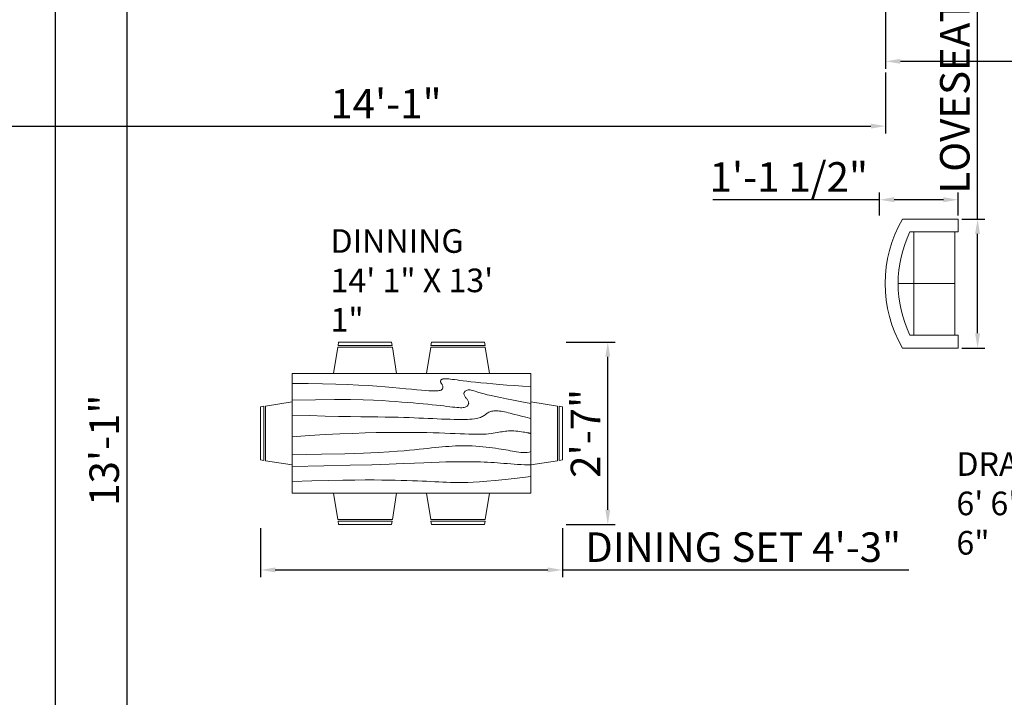
# Model space of a CAD drawing. Units: millimetres. Extents: x 2768 to 4359, y 795 to 1583.
# Tile 10 of 13: x 3764 to 3930, y 1258 to 1373. Entities that reach past the tile are written whole.
import ezdxf

# ---------------------------------------------------------------- set-up
doc = ezdxf.new("R2010")
doc.units = ezdxf.units.MM
for name, color, linetype, lineweight in [('A-ANNO-DIMS', 90, 'Continuous', 18), ('A-AREA-IDEN', 190, 'Continuous', 18), ('furniture', 50, 'Continuous', 18)]:
    doc.layers.add(name, color=color, linetype=linetype, lineweight=lineweight)
doc.styles.get("Standard").update_dxf_attribs({"font": 'arial.ttf'})
doc.dimstyles.new('ISO-25', dxfattribs={"dimtxt": 5, "dimasz": 2.5, "dimexe": 1.25, "dimexo": 0.625, "dimtad": 1, "dimdec": 0, "dimlunit": 3, "dimtxsty": 'Standard', "dimcen": 2.5, "dimadec": 0, "dimazin": 0, "dimtfac": 1, "dimtdec": 0, "dimtmove": 0, "dimatfit": 3, "dimfxl": 1, "dimarcsym": 0})

# ---------------------------------------------------------------- blocks, each defined once
blk = doc.blocks.new('Sofa - Roundback Loveseat 5 ft.')
for p, q in [((0, -32.44198), (0, -5.99998)), ((-24, -33.99998), (-24, -11.46958)), ((-23.9998, -13.38178), (23.99986, -13.38178)), ((24.00004, -33.99998), (24.00004, -11.46958)), ((-24, -32.44198), (24.00004, -32.44198))]:
    blk.add_line(p, q)
for points in [[(-24, -33.99998), (-30, -33.99998), (-30, -7.99998)], [(30.00004, -7.99998), (30.00004, -33.99998), (24.00004, -33.99998)]]:
    blk.add_lwpolyline(points)
for centre, radius, start, end in [((0, -60.24998), 60.24998, 60.13715, 119.8628), ((0, -61.38438), 55.38444, 64.32083, 115.6792)]:
    blk.add_arc(centre, radius, start, end)
blk = doc.blocks.new('Dining Set - 36 x 72 in.')
for p, q in [((-22, 27.5), (-22.1562, 26.50042)), ((-22, 27.5), (-6, 27.5)), ((-5.8437, 26.49966), (-6, 27.5)), ((6, 27.5), (5.8438, 26.50042)), ((6, 27.5), (22, 27.5)), ((22.1563, 26.49966), (22, 27.5)), ((-22.2343, 26.00059), (-23.4847, 17.99762)), ((-22.2304, 26), (-5.7608, 26)), ((-5.8416, 26.5), (-22.1534, 26.5)), ((-4.5152, 17.99762), (-5.7655, 25.99926)), ((5.7657, 26.00059), (4.5153, 17.99762)), ((5.7696, 26), (22.2392, 26)), ((22.1584, 26.5), (5.8466, 26.5)), ((23.4848, 17.99762), (22.2345, 25.99926)), ((36, 18), (-36, 18)), ((-36, 18), (-36, -18)), ((36, -18), (36, 18)), ((-44.0006, 8.23428), (-35.9976, 9.48474)), ((44.0006, 8.23428), (35.9976, 9.48474)), ((-45.5, 8), (-44.5004, 8.15617)), ((-45.5, 8), (-45.5, -8)), ((-44.5, -8.15843), (-44.5, 8.15338)), ((-44, 8.23041), (-44, -8.23915)), ((44, 8.23041), (44, -8.23915)), ((44.5, -8.15843), (44.5, 8.15338)), ((45.5, 8), (44.5005, 8.15617)), ((45.5, 8), (45.5, -8)), ((-44.4997, -8.15631), (-45.5, -8)), ((-35.9976, -9.48476), (-43.9993, -8.2345)), ((35.9976, -9.48476), (43.9993, -8.2345)), ((44.4997, -8.15631), (45.5, -8)), ((-36, -18), (36, -18)), ((-22.2343, -26.0006), (-23.4847, -17.99762)), ((-4.5152, -17.99762), (-5.7655, -25.99928)), ((5.7657, -26.0006), (4.5153, -17.99762)), ((23.4848, -17.99762), (22.2345, -25.99928)), ((-22.2304, -26), (-5.7608, -26)), ((-22, -27.5), (-22.1562, -26.50044)), ((-5.8416, -26.5), (-22.1534, -26.5)), ((-5.8437, -26.49967), (-6, -27.5)), ((5.7696, -26), (22.2392, -26)), ((6, -27.5), (5.8438, -26.50044)), ((22.1584, -26.5), (5.8466, -26.5)), ((22.1563, -26.49967), (22, -27.5)), ((-22, -27.5), (-6, -27.5)), ((6, -27.5), (22, -27.5))]:
    blk.add_line(p, q)
for points in [[(-36, 15), (-31.1772, 14.97754), (-26.8079, 14.91406), (-22.8538, 14.81543), (-19.276, 14.6875), (-16.0362, 14.53613), (-13.0957, 14.36718), (-10.4159, 14.18652), (-7.9583, 14), (-5.6904, 13.81315), (-3.6035, 13.63021), (-1.6954, 13.45508), (0.0365, 13.29166), (1.5945, 13.14388), (2.9811, 13.01562), (4.1988, 12.9108), (5.25, 12.83333), (6.1393, 12.78613), (6.8802, 12.76823), (7.4883, 12.77767), (7.9792, 12.8125), (8.3685, 12.87077), (8.6719, 12.95052), (8.9049, 13.0498), (9.0833, 13.16666), (9.2205, 13.29899), (9.3216, 13.44401), (9.3895, 13.59879), (9.4271, 13.76041), (9.4373, 13.92594), (9.4232, 14.09245), (9.3875, 14.257), (9.3333, 14.41666), (9.2638, 14.56917), (9.1836, 14.71484), (9.0975, 14.85465), (9.0104, 14.98958), (8.9272, 15.1206), (8.8529, 15.2487), (8.7922, 15.37483), (8.75, 15.5), (8.7305, 15.62467), (8.7344, 15.74739), (8.7617, 15.86621), (8.8125, 15.97916), (8.8867, 16.08431), (8.9844, 16.17968), (9.1055, 16.26334), (9.25, 16.33333), (9.4189, 16.38802), (9.6172, 16.42708), (9.8506, 16.45052), (10.125, 16.45833), (10.4463, 16.45052), (10.8203, 16.42708), (11.2529, 16.38802), (11.75, 16.33333), (12.3184, 16.26318), (12.9694, 16.17838), (13.7151, 16.07991), (14.5677, 15.96875), (15.5395, 15.84586), (16.6426, 15.71224), (17.8893, 15.56884), (19.2917, 15.41666), (20.859, 15.25667), (22.5879, 15.08984), (24.4721, 14.91715), (26.5052, 14.73958), (28.6809, 14.5581), (30.9929, 14.3737), (33.4347, 14.18733), (36, 14)], [(-36, 10), (-28.9766, 10.14274), (-23.1725, 10.20442), (-18.4241, 10.19775), (-14.5677, 10.13541), (-11.4399, 10.03011), (-8.877, 9.89453), (-6.7154, 9.74137), (-4.7917, 9.58333), (-2.9698, 9.43082), (-1.2246, 9.28515), (0.4415, 9.14534), (2.026, 9.01041), (3.5266, 8.87939), (4.9408, 8.7513), (6.266, 8.62516), (7.5, 8.5), (8.6411, 8.37549), (9.6914, 8.2539), (10.6538, 8.13818), (11.5312, 8.03125), (12.3267, 7.93603), (13.043, 7.85547), (13.6831, 7.79248), (14.25, 7.75), (14.7471, 7.7303), (15.1797, 7.73307), (15.5537, 7.75732), (15.875, 7.80208), (16.1494, 7.86637), (16.3828, 7.94922), (16.5811, 8.04964), (16.75, 8.16666), (16.8944, 8.29915), (17.0143, 8.44531), (17.1089, 8.60319), (17.1771, 8.77083), (17.218, 8.94629), (17.2305, 9.1276), (17.2137, 9.31282), (17.1667, 9.5), (17.0895, 9.6875), (16.987, 9.875), (16.8649, 10.0625), (16.7292, 10.25), (16.5856, 10.4375), (16.4401, 10.625), (16.2985, 10.8125), (16.1667, 11), (16.05, 11.18733), (15.9518, 11.3737), (15.8752, 11.5581), (15.8229, 11.73958), (15.798, 11.91715), (15.8034, 12.08984), (15.842, 12.25667), (15.9167, 12.41666), (16.0295, 12.56836), (16.1784, 12.70833), (16.3605, 12.83268), (16.5729, 12.9375), (16.8127, 13.01888), (17.0768, 13.07291), (17.3625, 13.0957), (17.6667, 13.08333), (17.9894, 13.03312), (18.3418, 12.94726), (18.7382, 12.82918), (19.1927, 12.68229), (19.7195, 12.51001), (20.3327, 12.31575), (21.0465, 12.10294), (21.875, 11.875), (22.8357, 11.63354), (23.959, 11.37304), (25.2786, 11.08618), (26.8282, 10.76562), (28.6414, 10.40405), (30.752, 9.99414), (33.1936, 9.52856), (36, 9)], [(-36, 5.5), (-30.7157, 5.3348), (-26.069, 5.20963), (-21.9946, 5.11767), (-18.4271, 5.05208), (-15.3009, 5.00602), (-12.5508, 4.97265), (-10.1112, 4.94515), (-7.9167, 4.91666), (-5.909, 4.88167), (-4.0586, 4.83984), (-2.3429, 4.79215), (-0.7396, 4.73958), (0.7739, 4.6831), (2.22, 4.6237), (3.6213, 4.56233), (5, 4.5), (6.373, 4.43782), (7.7344, 4.3776), (9.0723, 4.32129), (10.375, 4.27083), (11.6309, 4.22819), (12.8281, 4.19531), (13.9551, 4.17415), (15, 4.16666), (15.954, 4.17448), (16.819, 4.19791), (17.6001, 4.23698), (18.3021, 4.29166), (18.9299, 4.36198), (19.4883, 4.44791), (19.9823, 4.54948), (20.4167, 4.66666), (20.7969, 4.79899), (21.1302, 4.94401), (21.4245, 5.09879), (21.6875, 5.26041), (21.9271, 5.42594), (22.1511, 5.59245), (22.3672, 5.757), (22.5834, 5.91666), (22.8065, 6.06868), (23.0404, 6.21093), (23.2879, 6.34147), (23.5521, 6.45833), (23.8358, 6.55957), (24.142, 6.64323), (24.4735, 6.70735), (24.8334, 6.75), (25.2235, 6.76969), (25.642, 6.76692), (26.0858, 6.74267), (26.5521, 6.69791), (27.0379, 6.63362), (27.5404, 6.55078), (28.0565, 6.45036), (28.5834, 6.33333), (29.1242, 6.19987), (29.7071, 6.04687), (30.3661, 5.87044), (31.1354, 5.66666), (32.0493, 5.43164), (33.142, 5.16146), (34.4475, 4.85221), (36, 4.5)], [(-36, -1), (-30.7915, -0.6591), (-26.0195, -0.38216), (-21.6519, -0.16284), (-17.6563, 0.00521), (-14.0005, 0.12833), (-10.6523, 0.21289), (-7.5796, 0.26522), (-4.75, 0.29166), (-2.134, 0.29793), (0.2878, 0.28711), (2.5317, 0.26163), (4.6146, 0.22396), (6.5529, 0.17651), (8.3633, 0.12174), (10.0623, 0.06209), (11.6667, 0), (13.1899, -0.06201), (14.6341, -0.1211), (15.9982, -0.17432), (17.2813, -0.21875), (18.4823, -0.25147), (19.6003, -0.26953), (20.6343, -0.27002), (21.5834, -0.25), (22.4481, -0.20768), (23.2357, -0.14584), (23.9549, -0.06836), (24.6146, 0.02083), (25.2235, 0.11784), (25.7904, 0.21875), (26.3241, 0.31966), (26.8334, 0.41666), (27.3265, 0.50618), (27.8099, 0.58593), (28.2894, 0.65397), (28.7709, 0.70833), (29.2601, 0.74707), (29.763, 0.76823), (30.2855, 0.76985), (30.8334, 0.75), (31.4088, 0.70784), (31.9994, 0.64713), (32.589, 0.57275), (33.1615, 0.48958), (33.7008, 0.4025), (34.1908, 0.3164), (34.6153, 0.23616), (34.9584, 0.16666), (35.2099, 0.11165), (35.3848, 0.07031), (35.504, 0.04069), (35.5886, 0.02083), (35.6594, 0.00879), (35.7377, 0.0026), (35.8442, 0.00032), (36, 0)], [(-36, -6.5), (-27.1843, -6.31267), (-20.084, -6.1263), (-14.469, -5.9419), (-10.1094, -5.76042), (-6.7752, -5.58285), (-4.2363, -5.41016), (-2.2629, -5.24333), (-0.625, -5.08334), (0.8708, -4.93099), (2.2715, -4.78646), (3.5872, -4.64974), (4.8281, -4.52084), (6.0046, -4.39974), (7.127, -4.28646), (8.2053, -4.18099), (9.25, -4.08334), (10.2705, -3.99382), (11.2734, -3.91407), (12.2647, -3.84603), (13.25, -3.79167), (14.2354, -3.75293), (15.2266, -3.73177), (16.2295, -3.73015), (17.25, -3.75), (18.2912, -3.79248), (19.3451, -3.85547), (20.4009, -3.93604), (21.4479, -4.03125), (22.4754, -4.13819), (23.4727, -4.25391), (24.4289, -4.37549), (25.3334, -4.5), (26.1785, -4.62492), (26.9694, -4.74935), (27.7145, -4.87281), (28.4219, -4.99479), (29.1, -5.11483), (29.7572, -5.23242), (30.4016, -5.34709), (31.0417, -5.45834), (31.6837, -5.56437), (32.3262, -5.65821), (32.9658, -5.73153), (33.599, -5.77604), (34.2224, -5.78345), (34.8327, -5.74545), (35.4264, -5.65373), (36, -5.5)], [(-36, -10), (-26.4022, -9.81299), (-18.4675, -9.62891), (-11.9839, -9.45069), (-6.7396, -9.28125), (-2.5226, -9.12354), (0.8789, -8.98047), (3.6769, -8.85498), (6.0833, -8.75), (8.2767, -8.66765), (10.3021, -8.60677), (12.1712, -8.56543), (13.8958, -8.54167), (15.4876, -8.53353), (16.9583, -8.53907), (18.3197, -8.55632), (19.5834, -8.58334), (20.7616, -8.61841), (21.8685, -8.66081), (22.9188, -8.71004), (23.9271, -8.76563), (24.9081, -8.82707), (25.8763, -8.89388), (26.8465, -8.96558), (27.8334, -9.04167), (28.8474, -9.12118), (29.8828, -9.20117), (30.93, -9.27824), (31.9792, -9.34896), (33.0205, -9.40991), (34.0443, -9.45768), (35.0407, -9.48885), (36, -9.5)], [(-36, -14.5), (-30.0881, -14.33513), (-25.0332, -14.21224), (-20.7312, -14.12647), (-17.0781, -14.07292), (-13.97, -14.04671), (-11.3027, -14.04297), (-8.9724, -14.05681), (-6.875, -14.08334), (-4.9224, -14.11833), (-3.0905, -14.16016), (-1.3709, -14.20785), (0.2448, -14.26042), (1.7647, -14.3169), (3.1973, -14.3763), (4.5507, -14.43767), (5.8333, -14.5), (7.0554, -14.5621), (8.235, -14.62175), (9.3922, -14.67652), (10.5469, -14.72396), (11.7192, -14.76164), (12.929, -14.78711), (14.1965, -14.79794), (15.5417, -14.79167), (16.9933, -14.76424), (18.6152, -14.70508), (20.4804, -14.60197), (22.6615, -14.44271), (25.2312, -14.21509), (28.2624, -13.9069), (31.8277, -13.50594), (36, -13)]]:
    blk.add_lwpolyline(points)
blk = doc.blocks.new('*D63')
at = {"layer": 'A-ANNO-DIMS', "color": 0, "lineweight": -2, "transparency": 16777216}
for p, q in [((3910.37, 1378.18), (3910.37, 1364.91)), ((3988.37, 1378.18), (3988.37, 1364.91)), ((3912.87, 1366.16), (3985.87, 1366.16))]:
    blk.add_line(p, q, dxfattribs=at)
at = {"layer": 'A-ANNO-DIMS', "color": 0, "transparency": 16777216}
for points in [[(3912.87, 1366.57), (3912.87, 1365.74), (3910.37, 1366.16)], [(3985.87, 1366.57), (3985.87, 1365.74), (3988.37, 1366.16)]]:
    blk.add_solid(points, dxfattribs=at)
at = {"layer": 'Defpoints', "color": 0, "transparency": 16777216}
for p in [(3910.37, 1378.81), (3988.37, 1378.81), (3988.37, 1366.16)]:
    blk.add_point(p, dxfattribs=at)
at = {"layer": 'A-ANNO-DIMS', "color": 0, "transparency": 16777216, "insert": (3949.37, 1369.33), "char_height": 5, "attachment_point": 5}
blk.add_mtext('6\'-6"', dxfattribs=at)
blk = doc.blocks.new('*D64')
at = {"layer": 'A-ANNO-DIMS', "color": 0, "lineweight": -2, "transparency": 16777216}
for p, q in [((3910.37, 1364.28), (3910.37, 1353.94)), ((3741.08, 1357.5), (3741.08, 1353.94)), ((3743.58, 1355.19), (3907.87, 1355.19))]:
    blk.add_line(p, q, dxfattribs=at)
at = {"layer": 'A-ANNO-DIMS', "color": 0, "transparency": 16777216}
for points in [[(3743.58, 1355.61), (3743.58, 1354.77), (3741.08, 1355.19)], [(3907.87, 1355.61), (3907.87, 1354.77), (3910.37, 1355.19)]]:
    blk.add_solid(points, dxfattribs=at)
at = {"layer": 'Defpoints', "color": 0, "transparency": 16777216}
for p in [(3910.37, 1364.91), (3741.08, 1358.13), (3910.37, 1355.19)]:
    blk.add_point(p, dxfattribs=at)
at = {"layer": 'A-ANNO-DIMS', "color": 0, "transparency": 16777216, "insert": (3825.72, 1358.33), "char_height": 5, "attachment_point": 5}
blk.add_mtext('14\'-1"', dxfattribs=at)
blk = doc.blocks.new('*D65')
at = {"layer": 'A-ANNO-DIMS', "color": 0, "lineweight": -2, "transparency": 16777216}
for p, q in [((3776.14, 1378.81), (3783.06, 1378.81)), ((3781.81, 1376.31), (3781.81, 1224.31)), ((3776.14, 1221.81), (3783.06, 1221.81))]:
    blk.add_line(p, q, dxfattribs=at)
at = {"layer": 'A-ANNO-DIMS', "color": 0, "transparency": 16777216}
for points in [[(3781.39, 1376.31), (3782.23, 1376.31), (3781.81, 1378.81)], [(3781.39, 1224.31), (3782.23, 1224.31), (3781.81, 1221.81)]]:
    blk.add_solid(points, dxfattribs=at)
at = {"layer": 'Defpoints', "color": 0, "transparency": 16777216}
for p in [(3775.51, 1378.81), (3775.51, 1221.81), (3781.81, 1221.81)]:
    blk.add_point(p, dxfattribs=at)
at = {"layer": 'A-ANNO-DIMS', "color": 0, "transparency": 16777216, "insert": (3778.63, 1300.31), "char_height": 5, "attachment_point": 5, "rotation": 90}
blk.add_mtext('13\'-1"', dxfattribs=at)
blk = doc.blocks.new('*D111')
at = {"layer": 'A-ANNO-DIMS', "color": 0, "lineweight": -2, "transparency": 16777216}
for p, q in [((3925.95, 1339.44), (3925.95, 1398.97)), ((3923.3, 1339.44), (3927.2, 1339.44)), ((3925.95, 1320.11), (3925.95, 1336.94)), ((3923.3, 1317.61), (3927.2, 1317.61))]:
    blk.add_line(p, q, dxfattribs=at)
at = {"layer": 'A-ANNO-DIMS', "color": 0, "transparency": 16777216}
for points in [[(3925.53, 1336.94), (3926.37, 1336.94), (3925.95, 1339.44)], [(3925.53, 1320.11), (3926.37, 1320.11), (3925.95, 1317.61)]]:
    blk.add_solid(points, dxfattribs=at)
at = {"layer": 'Defpoints', "color": 0, "transparency": 16777216}
for p in [(3922.67, 1339.44), (3925.95, 1339.44), (3922.67, 1317.61)]:
    blk.add_point(p, dxfattribs=at)
at = {"layer": 'A-ANNO-DIMS', "color": 0, "transparency": 16777216, "insert": (3922.74, 1370.46), "char_height": 5, "attachment_point": 5, "rotation": 90}
blk.add_mtext('LOVESEAT 1\'-10"', dxfattribs=at)
blk = doc.blocks.new('*D112')
at = {"layer": 'A-ANNO-DIMS', "color": 0, "lineweight": -2, "transparency": 16777216}
for p, q in [((3909.33, 1340.07), (3909.33, 1343.97)), ((3922.67, 1340.07), (3922.67, 1343.97)), ((3909.33, 1342.72), (3881.11, 1342.72)), ((3920.17, 1342.72), (3911.83, 1342.72))]:
    blk.add_line(p, q, dxfattribs=at)
at = {"layer": 'A-ANNO-DIMS', "color": 0, "transparency": 16777216}
for points in [[(3911.83, 1343.14), (3911.83, 1342.3), (3909.33, 1342.72)], [(3920.17, 1343.14), (3920.17, 1342.3), (3922.67, 1342.72)]]:
    blk.add_solid(points, dxfattribs=at)
at = {"layer": 'Defpoints', "color": 0, "transparency": 16777216}
for p in [(3909.33, 1342.72), (3909.33, 1339.44), (3922.67, 1339.44)]:
    blk.add_point(p, dxfattribs=at)
at = {"layer": 'A-ANNO-DIMS', "color": 0, "transparency": 16777216, "insert": (3893.97, 1345.93), "char_height": 5, "attachment_point": 5}
blk.add_mtext('1\'-1 1/2"', dxfattribs=at)
blk = doc.blocks.new('*D123')
at = {"layer": 'A-ANNO-DIMS', "color": 0, "lineweight": -2, "transparency": 16777216}
for p, q in [((3804.47, 1287.08), (3804.47, 1278.78)), ((3855.62, 1287.08), (3855.62, 1278.78)), ((3806.97, 1280.03), (3853.12, 1280.03)), ((3855.62, 1280.03), (3914.33, 1280.03))]:
    blk.add_line(p, q, dxfattribs=at)
at = {"layer": 'A-ANNO-DIMS', "color": 0, "transparency": 16777216}
for points in [[(3806.97, 1280.45), (3806.97, 1279.62), (3804.47, 1280.03)], [(3853.12, 1280.45), (3853.12, 1279.62), (3855.62, 1280.03)]]:
    blk.add_solid(points, dxfattribs=at)
at = {"layer": 'Defpoints', "color": 0, "transparency": 16777216}
for p in [(3804.47, 1287.71), (3855.62, 1287.71), (3855.62, 1280.03)]:
    blk.add_point(p, dxfattribs=at)
at = {"layer": 'A-ANNO-DIMS', "color": 0, "transparency": 16777216, "insert": (3886.23, 1283.24), "char_height": 5, "attachment_point": 5}
blk.add_mtext('DINING SET 4\'-3"', dxfattribs=at)
blk = doc.blocks.new('*D124')
at = {"layer": 'A-ANNO-DIMS', "color": 0, "lineweight": -2, "transparency": 16777216}
for p, q in [((3856.25, 1318.62), (3864.55, 1318.62)), ((3863.3, 1290.21), (3863.3, 1316.12)), ((3856.25, 1287.71), (3864.55, 1287.71))]:
    blk.add_line(p, q, dxfattribs=at)
at = {"layer": 'A-ANNO-DIMS', "color": 0, "transparency": 16777216}
for points in [[(3862.88, 1316.12), (3863.71, 1316.12), (3863.3, 1318.62)], [(3862.88, 1290.21), (3863.71, 1290.21), (3863.3, 1287.71)]]:
    blk.add_solid(points, dxfattribs=at)
at = {"layer": 'Defpoints', "color": 0, "transparency": 16777216}
for p in [(3855.62, 1318.62), (3863.3, 1318.62), (3855.62, 1287.71)]:
    blk.add_point(p, dxfattribs=at)
at = {"layer": 'A-ANNO-DIMS', "color": 0, "transparency": 16777216, "insert": (3860.16, 1303.16), "char_height": 5, "attachment_point": 5, "rotation": 90}
blk.add_mtext('2\'-7"', dxfattribs=at)
blk = doc.blocks.new('*D135')
at = {"layer": 'A-ANNO-DIMS', "color": 0, "lineweight": -2, "transparency": 16777216}
for p, q in [((3741.08, 1378.18), (3741.08, 798.41)), ((3769.66, 1378.18), (3769.66, 798.41)), ((3743.58, 799.66), (3767.16, 799.66))]:
    blk.add_line(p, q, dxfattribs=at)
at = {"layer": 'A-ANNO-DIMS', "color": 0, "transparency": 16777216}
for points in [[(3743.58, 800.08), (3743.58, 799.24), (3741.08, 799.66)], [(3767.16, 800.08), (3767.16, 799.24), (3769.66, 799.66)]]:
    blk.add_solid(points, dxfattribs=at)
at = {"layer": 'Defpoints', "color": 0, "transparency": 16777216}
for p in [(3741.08, 1378.81), (3769.66, 1378.81), (3769.66, 799.66)]:
    blk.add_point(p, dxfattribs=at)
at = {"layer": 'A-ANNO-DIMS', "color": 0, "transparency": 16777216, "insert": (3755.37, 802.87), "char_height": 5, "attachment_point": 5}
blk.add_mtext('2\'-4 1/2"', dxfattribs=at)

msp = doc.modelspace()

# ---------------------------------------------------------------- block references
at = {"layer": 'furniture', "xscale": 0.3639013713455709, "yscale": 0.3639013713455709, "zscale": 0.3639013713455709, "rotation": 90}
msp.add_blockref('Sofa - Roundback Loveseat 5 ft.', (3910.3, 1328.53), dxfattribs=at)
at = {"layer": 'furniture', "xscale": 0.5621081790336501, "yscale": 0.5621081790336501, "zscale": 0.5621081790336501}
msp.add_blockref('Dining Set - 36 x 72 in.', (3830.05, 1303.16), dxfattribs=at)

# ---------------------------------------------------------------- texts
at = {"layer": 'A-AREA-IDEN', "char_height": 4, "attachment_point": 1}
for s, width, insert in [('DINNING \\P14\' 1" X 13\' 1"', 33.515, (3816.32, 1337.73)), ('DRAWING \\P6\' 6" X 11\' 6"', 29.6052, (3922.36, 1299.96))]:
    msp.add_mtext_dynamic_manual_height_columns(s, width=width, gutter_width=12.5, heights=[0], dxfattribs=dict(at, insert=insert))

# ---------------------------------------------------------------- dimensions: what is measured, and where the dimension line sits
at = {"layer": 'A-ANNO-DIMS'}
dim = msp.add_linear_dim(base=(3925.95, 1339.44), p1=(3922.67, 1317.61), p2=(3922.67, 1339.44), angle=90, text='LOVESEAT <>', dimstyle='ISO-25', override={"dimdec": 1, "dimlfac": 1, "dimrnd": 0, "dimzin": 1, "dimdsep": 46, "dimlunit": 4, "dimfrac": 2}, dxfattribs=at)
dim.commit()
dim.dimension.update_dxf_attribs({"geometry": '*D111', "text_midpoint": (3922.74, 1370.46)})
for base, p1, p2, override, picture, middle in [((3769.66, 799.66), (3741.08, 1378.81), (3769.66, 1378.81), {"dimdec": 1, "dimlfac": 1, "dimrnd": 0, "dimzin": 1, "dimdsep": 46, "dimlunit": 4, "dimfrac": 2}, '*D135', (3755.37, 802.87)), ((3988.37, 1366.16), (3910.37, 1378.81), (3988.37, 1378.81), {"dimclrd": 0, "dimclre": 0, "dimclrt": 0}, '*D63', (3949.37, 1369.33)), ((3910.37, 1355.19), (3741.08, 1358.13), (3910.37, 1364.91), {"dimclrd": 0, "dimclre": 0, "dimclrt": 0}, '*D64', (3825.72, 1358.33))]:
    dim = msp.add_linear_dim(base=base, p1=p1, p2=p2, dimstyle='ISO-25', override=override, dxfattribs=at)
    dim.commit()
    dim.dimension.update_dxf_attribs({"geometry": picture, "text_midpoint": middle})
for base, p1, p2, angle, override, picture, middle in [((3781.81, 1221.81), (3775.51, 1378.81), (3775.51, 1221.81), 90, {"dimclrd": 0, "dimclre": 0, "dimclrt": 0}, '*D65', (3778.63, 1300.31)), ((3909.33, 1342.72), (3922.67, 1339.44), (3909.33, 1339.44), 180, {"dimdec": 1, "dimlfac": 1, "dimrnd": 0, "dimzin": 1, "dimdsep": 46, "dimlunit": 4, "dimfrac": 2}, '*D112', (3893.97, 1345.93)), ((3863.3, 1318.62), (3855.62, 1287.71), (3855.62, 1318.62), 90, {"dimdec": 1, "dimlfac": 1, "dimrnd": 0, "dimzin": 1, "dimdsep": 46, "dimlunit": 4, "dimfrac": 2}, '*D124', (3860.16, 1303.16))]:
    dim = msp.add_linear_dim(base=base, p1=p1, p2=p2, angle=angle, dimstyle='ISO-25', override=override, dxfattribs=at)
    dim.commit()
    dim.dimension.update_dxf_attribs({"geometry": picture, "text_midpoint": middle})
dim = msp.add_linear_dim(base=(3855.6239, 1280.0328), p1=(3804.472, 1287.7056), p2=(3855.6239, 1287.7056), text='DINING SET <>', dimstyle='ISO-25', override={"dimdec": 1, "dimlfac": 1, "dimrnd": 0, "dimzin": 1, "dimdsep": 46, "dimlunit": 4, "dimfrac": 2}, dxfattribs=at)
dim.commit()
dim.dimension.update_dxf_attribs({"geometry": '*D123', "text_midpoint": (3886.2267, 1283.2448)})

doc.saveas('drawing.dxf')
